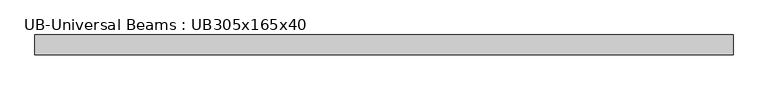
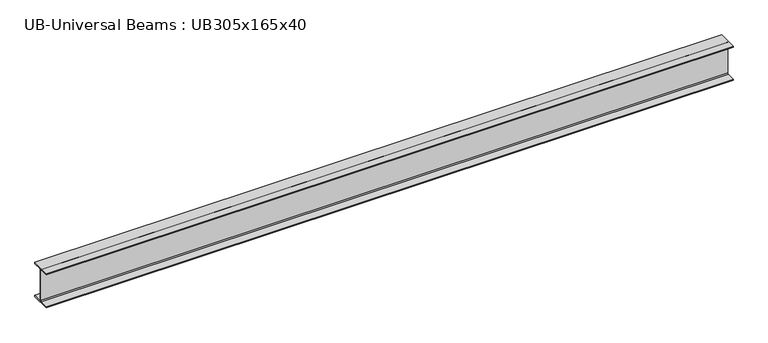
"""IFC4 building model written with IfcOpenShell, lengths in millimetres: beam geometry, UB-Universal Beams : UB305x165x40."""

from ifc_helpers import new_model, si_unit, point, frame, frame_2d, origin, place, context, project, spatial, polyline, circle_curve, trimmed, segment, composite_curve, outline, extrude, source, transform, mapped, element, save


def ub_universal_beams_ub305x165x40_616d6e4e(model_context):
    return source(origin(), model_context, "Body", "SweptSolid", [
        extrude(outline(composite_curve([segment(polyline([(82.5, -141.5), (82.5, -151.7), (-82.5, -151.7), (-82.5, -141.5), (-11.9, -141.5)]), True, "CONTINUOUS"), segment(trimmed(circle_curve(frame_2d((-11.9, -132.6)), 8.9), [point((-11.9, -141.5))], [point((-3.0, -132.6))], True, "CARTESIAN"), True, "CONTINUOUS"), segment(polyline([(-3.0, -132.6), (-3.0, 132.6)]), True, "CONTINUOUS"), segment(trimmed(circle_curve(frame_2d((-11.9, 132.6)), 8.9), [point((-3.0, 132.6))], [point((-11.9, 141.5))], True, "CARTESIAN"), True, "CONTINUOUS"), segment(polyline([(-11.9, 141.5), (-82.5, 141.5), (-82.5, 151.7), (82.5, 151.7), (82.5, 141.5), (11.9, 141.5)]), True, "CONTINUOUS"), segment(trimmed(circle_curve(frame_2d((11.9, 132.6)), 8.9), [point((11.9, 141.5))], [point((3.0, 132.6))], True, "CARTESIAN"), True, "CONTINUOUS"), segment(polyline([(3.0, 132.6), (3.0, -132.6)]), True, "CONTINUOUS"), segment(trimmed(circle_curve(frame_2d((11.9, -132.6)), 8.9), [point((3.0, -132.6))], [point((11.9, -141.5))], True, "CARTESIAN"), True, "CONTINUOUS"), segment(polyline([(11.9, -141.5), (82.5, -141.5)]), True, "CONTINUOUS")], self_intersect=False)), frame((-2882.6, 0.0, 0.0), z_axis=(1.0, 0.0, 0.0), x_axis=(0.0, 1.0, 0.0)), (0.0, 0.0, 1.0), 5765.2),
    ])


if __name__ == "__main__":
    model = new_model("IFC4")
    model_context = context("Model", 3, world=origin())
    ifc_project = project(units=[si_unit("LENGTHUNIT", "METRE", prefix="MILLI")], contexts=[model_context])
    site = spatial("IfcSite", under=ifc_project)
    building = spatial("IfcBuilding", under=site)
    placement = place(None, origin())
    ub_universal_beams_ub305x165x40_shape = ub_universal_beams_ub305x165x40_616d6e4e(model_context)
    element("IfcBeam", 1, ObjectType="UB-Universal Beams : UB305x165x40", at=placement, inside=building, context=model_context, shape_type="MappedRepresentation", body=[
        mapped(ub_universal_beams_ub305x165x40_shape, transform((0.0, 0.0, 0.0), x_axis=(1.0, 0.0, 0.0), y_axis=(0.0, 1.0, 0.0), z_axis=(0.0, 0.0, 1.0))),
    ])
    save(model, "model.ifc")

# Revit data of these elements
# Type "UB-Universal Beams : UB305x165x40"
#   Section Name Key = "UB305X165X40"
#   Width = 16.5 cm
#   Web Thickness = 0.6 cm
#   Web Fillet = 0.89 cm
#   Warping Constant = 164000.0 cm⁶
#   Torsional Moment of Inertia = 14.70 cm⁴
#   Section Area = 51.3 cm²
#   Plastic Modulus weak axis = 142.0 cm³
#   Plastic Modulus strong axis = 623.0 cm³
#   Nominal Weight = 40.2999 kgf/m
#   Moment of Inertia weak axis = 764.00 cm⁴
#   Moment of Inertia strong axis = 8503.00 cm⁴
#   Height = 30.34 cm
#   Flange Thickness = 1.02 cm
#   Elastic Modulus weak axis = 92.6 cm³
#   Elastic Modulus strong axis = 560.0 cm³
#   Centroid Vertical = 15.17 cm
#   Centroid Horizontal = 8.25 cm
#   Bolt Spacing = 9.0 cm
#   Length [instance default] = 1500 mm
#   Structural Material [instance default] = Metal - Steel 43-275
#   Type Comments = ""
#   Assembly Code = ""
# Element 1 (IfcBeam, "UB-Universal Beams : UB305x165x40")
#   Materials on its faces: "Metal - Steel 43-275"
# Materials
#   "Metal - Steel 43-275": class "Metal", colour RGB 247 247 247, transparency 0, Cost = 0
